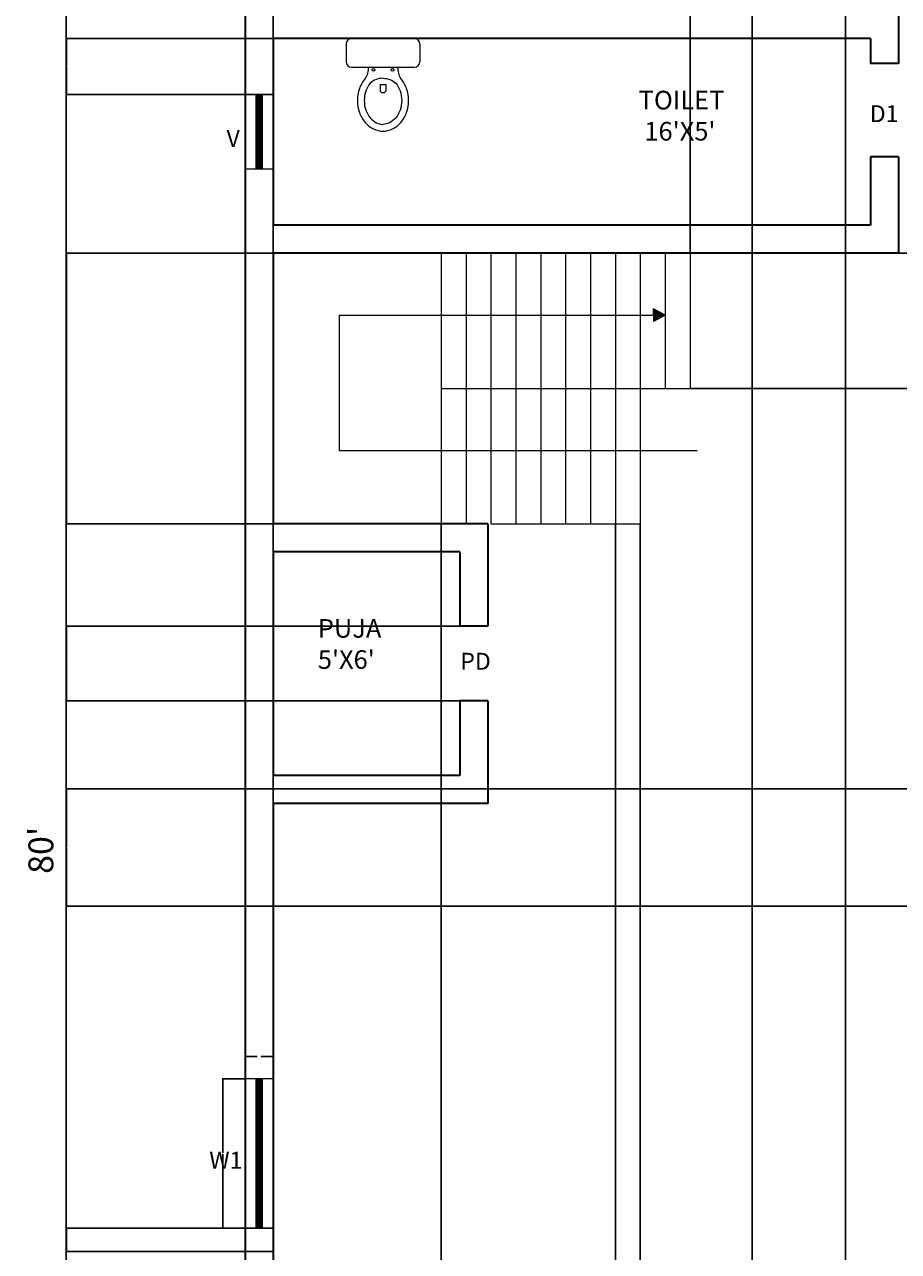
# Model space of a CAD drawing. Units: inches. Extents: x 318 to 927, y -1130 to 13.
# Tile 8 of 17: x 318 to 599, y -692 to -297. Entities that reach past the tile are written whole.
import ezdxf

# ---------------------------------------------------------------- set-up
doc = ezdxf.new("R2010")
doc.units = ezdxf.units.IN
doc.header["$MEASUREMENT"] = 0
for name, color, linetype, lineweight in [('A-ANNO-DIMS', 1, 'Continuous', 18), ('A-ANNO-IDEN', 1, 'Continuous', 13), ('A-ANNO-SYMB', 1, 'Continuous', 13), ('A-AREA-IDEN', 8, 'Continuous', 18), ('A-FLOR-FIXT', 7, 'Continuous', 18), ('A-FLOR-STRS', 1, 'Continuous', 18), ('A-GLAZ-PATT', 5, 'Continuous', 9), ('wall', 1, 'Continuous', 35), ('win', 5, 'Continuous', 18)]:
    doc.layers.add(name, color=color, linetype=linetype, lineweight=lineweight)
doc.styles.get("Standard").update_dxf_attribs({"font": 'arial.ttf'})
doc.dimstyles.get("Standard").update_dxf_attribs({"dimtxt": 0.18, "dimasz": 0.18, "dimexe": 0.18, "dimexo": 0.0625, "dimgap": 0.09, "dimtad": 0, "dimtih": 1, "dimtoh": 1, "dimdec": 1, "dimzin": 0, "dimdsep": 46, "dimlunit": 4, "dimtxsty": 'Standard', "dimcen": 0.09, "dimadec": 0, "dimazin": 0, "dimtfac": 1, "dimtdec": 1, "dimtofl": 0, "dimtmove": 0, "dimatfit": 3, "dimfxl": 1, "dimtolj": 1, "dimtzin": 0, "dimarcsym": 0})

# ---------------------------------------------------------------- blocks, each defined once
blk = doc.blocks.new('WC-P01')
for p, q in [((-230, 0), (230, 0)), ((-270, -40), (-270, -170)), ((270, -40), (270, -170)), ((-230, -210), (230, -210)), ((-111.4, -210), (-111.4, -210)), ((-20, -337.8), (20, -337.8)), ((-20, -337.8), (-20, -385.7)), ((20, -337.8), (20, -385.7)), ((-18.5, -389.3), (-10.5, -397.3)), ((-10.5, -397.3), (10.5, -397.3)), ((10.5, -397.3), (18.5, -389.3))]:
    blk.add_line(p, q)
for points in [[(-111.4, -210, -0.215497), (-132.6, -295.9, 0.09084), (-172.8, -367.1, 0.083285), (-187.5, -455, 0.083285), (-172.8, -542.9, 0.09084), (-132.6, -614.1, 0.104065), (-70, -663.6, 0.115836), (0, -680, 0.115836), (70, -663.6, 0.104065), (132.6, -614.1, 0.09084), (172.8, -542.9, 0.083285), (187.5, -455, 0.083285)], [(-70, -246.4), (-70, -246.4, 0.104065)], [(70, -246.4), (70, -246.4, 0.115836)], [(187.5, -455, 0.083285), (172.8, -367.1, 0.09084), (132.6, -295.9, -0.156524), (111.4, -210)], [(-1.8, -291.3, 0.171753), (-94.2, -327.9, 0.09084), (-125.5, -383.5, 0.083285), (-137.5, -455, 0.083285), (-125.5, -526.5, 0.09084), (-94.2, -582.1, 0.104065), (-47.7, -618.8, 0.115836), (0, -630, 0.115836)], [(1.8, -291.3, -0.171753), (94.2, -327.9, -0.09084), (125.5, -383.5, -0.083285), (137.5, -455, -0.083285), (125.5, -526.5, -0.09084), (94.2, -582.1, -0.104065), (47.7, -618.8, -0.115836), (0, -630, -0.115836)]]:
    blk.add_lwpolyline(points, format="xyb")
for centre in [(-70, -230), (70, -230)]:
    blk.add_circle(centre, 10)
for centre, radius, start, end in [((-230, -40), 40, 90, 180), ((230, -40), 40, 0, 90), ((-230, -170), 40, 180, 270), ((230, -170), 40, 270, 0), ((-15, -385.7), 5, 180, 225), ((15, -385.7), 5, 315, 0)]:
    blk.add_arc(centre, radius, start, end)
blk = doc.blocks.new('_ArchTick')
at = {"color": 0, "linetype": 'ByBlock', "const_width": 0.15}
blk.add_lwpolyline([(-0.5, -0.5), (0.5, 0.5)], dxfattribs=at)
blk = doc.blocks.new('*D4')
at = {"layer": 'A-ANNO-DIMS', "color": 0, "lineweight": -2, "transparency": 16777216}
blk.add_line((331.26, -82.91), (331.26, -1042.91), dxfattribs=at)
at = {"layer": 'Defpoints', "color": 0, "transparency": 16777216}
for p in [(388.89, -82.91), (331.26, -1042.91), (388.89, -1042.91)]:
    blk.add_point(p, dxfattribs=at)
at = {"layer": 'A-ANNO-DIMS', "color": 0, "lineweight": -2, "transparency": 16777216, "xscale": 6, "yscale": 6, "zscale": 6}
for p, rotation in [((331.26, -82.91), 90), ((331.26, -1042.91), 270)]:
    blk.add_blockref('_ArchTick', p, dxfattribs=dict(at, rotation=rotation))
at = {"layer": 'A-ANNO-DIMS', "color": 0, "transparency": 16777216, "insert": (323.18, -562.91), "char_height": 8, "attachment_point": 5, "rotation": 90}
blk.add_mtext("\\A1;80'", dxfattribs=at)
blk = doc.blocks.new('WIN-48IN')
for p, q in [((0, 48), (9, 48)), ((3.5, 48), (3.5, 0)), ((5.5, 48), (5.5, 0)), ((0, 0), (9, 0))]:
    blk.add_line(p, q)
blk = doc.blocks.new('VENT-24IN')
for p, q in [((9, 24), (0, 24)), ((3.5, 0), (3.5, 24)), ((5.5, 0), (5.5, 24)), ((9, 0), (0, 0))]:
    blk.add_line(p, q)
blk = doc.blocks.new('*D19')
at = {"layer": 'A-ANNO-DIMS', "color": 0, "lineweight": -2, "transparency": 16777216}
for p, q in [((388.83, -636.41), (381.51, -636.41)), ((381.69, -636.59), (381.69, -660.23)), ((381.69, -684.23), (381.69, -660.6)), ((388.83, -684.41), (381.51, -684.41))]:
    blk.add_line(p, q, dxfattribs=at)
at = {"layer": 'A-ANNO-DIMS', "color": 0, "transparency": 16777216}
for points in [[(381.66, -636.59), (381.72, -636.59), (381.69, -636.41)], [(381.66, -684.23), (381.72, -684.23), (381.69, -684.41)]]:
    blk.add_solid(points, dxfattribs=at)
at = {"layer": 'Defpoints', "color": 0, "transparency": 16777216}
for p in [(388.89, -636.41), (381.69, -684.41), (388.89, -684.41)]:
    blk.add_point(p, dxfattribs=at)
at = {"layer": 'A-ANNO-DIMS', "color": 0, "transparency": 16777216, "insert": (381.69, -660.41), "char_height": 0.18, "attachment_point": 5}
blk.add_mtext('\\A1;WINDOW W1 4\'-0" TYP.', dxfattribs=at)
blk = doc.blocks.new('*D20')
at = {"layer": 'A-ANNO-DIMS', "color": 0, "lineweight": -2, "transparency": 16777216}
for p, q in [((388.89, -636.35), (388.89, -629.03)), ((389.07, -629.21), (392.76, -629.21)), ((397.71, -629.21), (394.03, -629.21)), ((397.89, -636.35), (397.89, -629.03))]:
    blk.add_line(p, q, dxfattribs=at)
at = {"layer": 'A-ANNO-DIMS', "color": 0, "transparency": 16777216}
for points in [[(389.07, -629.18), (389.07, -629.24), (388.89, -629.21)], [(397.71, -629.18), (397.71, -629.24), (397.89, -629.21)]]:
    blk.add_solid(points, dxfattribs=at)
at = {"layer": 'Defpoints', "color": 0, "transparency": 16777216}
for p in [(388.89, -629.21), (388.89, -636.41), (397.89, -636.41)]:
    blk.add_point(p, dxfattribs=at)
at = {"layer": 'A-ANNO-DIMS', "color": 0, "transparency": 16777216, "insert": (393.39, -629.21), "char_height": 0.18, "attachment_point": 5}
blk.add_mtext('\\A1;0\'-9" TYP.', dxfattribs=at)
blk = doc.blocks.new('*D30')
at = {"layer": 'A-ANNO-DIMS', "color": 0, "lineweight": -2, "transparency": 16777216}
for p, q in [((551.89, -820.85), (551.89, -25.23)), ((552.07, -25.41), (566.56, -25.41)), ((581.71, -25.41), (567.23, -25.41)), ((581.89, -820.85), (581.89, -25.23))]:
    blk.add_line(p, q, dxfattribs=at)
at = {"layer": 'A-ANNO-DIMS', "color": 0, "transparency": 16777216}
for points in [[(552.07, -25.38), (552.07, -25.44), (551.89, -25.41)], [(581.71, -25.38), (581.71, -25.44), (581.89, -25.41)]]:
    blk.add_solid(points, dxfattribs=at)
at = {"layer": 'Defpoints', "color": 0, "transparency": 16777216}
for p in [(581.89, -25.41), (551.89, -820.91), (581.89, -820.91)]:
    blk.add_point(p, dxfattribs=at)
at = {"layer": 'A-ANNO-DIMS', "color": 0, "transparency": 16777216, "insert": (566.89, -25.41), "char_height": 0.18, "attachment_point": 5}
blk.add_mtext('\\A1;2\'-6"', dxfattribs=at)
blk = doc.blocks.new('*D32')
at = {"layer": 'A-ANNO-DIMS', "color": 0, "lineweight": -2, "transparency": 16777216}
for p, q in [((457.83, -490.91), (331.21, -490.91)), ((331.39, -491.09), (331.39, -502.73)), ((331.39, -514.73), (331.39, -503.09)), ((457.83, -514.91), (331.21, -514.91))]:
    blk.add_line(p, q, dxfattribs=at)
at = {"layer": 'A-ANNO-DIMS', "color": 0, "transparency": 16777216}
for points in [[(331.36, -491.09), (331.42, -491.09), (331.39, -490.91)], [(331.36, -514.73), (331.42, -514.73), (331.39, -514.91)]]:
    blk.add_solid(points, dxfattribs=at)
at = {"layer": 'Defpoints', "color": 0, "transparency": 16777216}
for p in [(457.89, -490.91), (331.39, -514.91), (457.89, -514.91)]:
    blk.add_point(p, dxfattribs=at)
at = {"layer": 'A-ANNO-DIMS', "color": 0, "transparency": 16777216, "insert": (331.39, -502.91), "char_height": 0.18, "attachment_point": 5}
blk.add_mtext('\\A1;2\'-0"', dxfattribs=at)
blk = doc.blocks.new('*D33')
at = {"layer": 'A-ANNO-DIMS', "color": 0, "lineweight": -2, "transparency": 16777216}
for p, q in [((397.89, -370.85), (397.89, -25.23)), ((398.07, -25.41), (464.5, -25.41)), ((531.71, -25.41), (465.28, -25.41)), ((531.89, -370.85), (531.89, -25.23))]:
    blk.add_line(p, q, dxfattribs=at)
at = {"layer": 'A-ANNO-DIMS', "color": 0, "transparency": 16777216}
for points in [[(398.07, -25.38), (398.07, -25.44), (397.89, -25.41)], [(531.71, -25.38), (531.71, -25.44), (531.89, -25.41)]]:
    blk.add_solid(points, dxfattribs=at)
at = {"layer": 'Defpoints', "color": 0, "transparency": 16777216}
for p in [(531.89, -25.41), (397.89, -370.91), (531.89, -370.91)]:
    blk.add_point(p, dxfattribs=at)
at = {"layer": 'A-ANNO-DIMS', "color": 0, "transparency": 16777216, "insert": (464.89, -25.41), "char_height": 0.18, "attachment_point": 5}
blk.add_mtext('\\A1;11\'-2"', dxfattribs=at)
blk = doc.blocks.new('*D34')
at = {"layer": 'A-ANNO-DIMS', "color": 0, "lineweight": -2, "transparency": 16777216}
for p, q in [((397.83, -370.91), (331.21, -370.91)), ((331.39, -371.09), (331.39, -414.23)), ((331.39, -457.73), (331.39, -414.59)), ((397.83, -457.91), (331.21, -457.91))]:
    blk.add_line(p, q, dxfattribs=at)
at = {"layer": 'A-ANNO-DIMS', "color": 0, "transparency": 16777216}
for points in [[(331.36, -371.09), (331.42, -371.09), (331.39, -370.91)], [(331.36, -457.73), (331.42, -457.73), (331.39, -457.91)]]:
    blk.add_solid(points, dxfattribs=at)
at = {"layer": 'Defpoints', "color": 0, "transparency": 16777216}
for p in [(397.89, -370.91), (331.39, -457.91), (397.89, -457.91)]:
    blk.add_point(p, dxfattribs=at)
at = {"layer": 'A-ANNO-DIMS', "color": 0, "transparency": 16777216, "insert": (331.39, -414.41), "char_height": 0.18, "attachment_point": 5}
blk.add_mtext('\\A1;7\'-3"', dxfattribs=at)
blk = doc.blocks.new('*D35')
at = {"layer": 'A-ANNO-DIMS', "color": 0, "lineweight": -2, "transparency": 16777216}
for p, q in [((397.89, -457.98), (397.89, -1124.59)), ((451.89, -457.98), (451.89, -1124.59)), ((398.07, -1124.41), (424.56, -1124.41)), ((451.71, -1124.41), (425.23, -1124.41))]:
    blk.add_line(p, q, dxfattribs=at)
at = {"layer": 'A-ANNO-DIMS', "color": 0, "transparency": 16777216}
for points in [[(398.07, -1124.38), (398.07, -1124.44), (397.89, -1124.41)], [(451.71, -1124.38), (451.71, -1124.44), (451.89, -1124.41)]]:
    blk.add_solid(points, dxfattribs=at)
at = {"layer": 'Defpoints', "color": 0, "transparency": 16777216}
for p in [(397.89, -457.91), (451.89, -457.91), (451.89, -1124.41)]:
    blk.add_point(p, dxfattribs=at)
at = {"layer": 'A-ANNO-DIMS', "color": 0, "transparency": 16777216, "insert": (424.89, -1124.41), "char_height": 0.18, "attachment_point": 5}
blk.add_mtext('\\A1;4\'-6"', dxfattribs=at)
blk = doc.blocks.new('*D36')
at = {"layer": 'A-ANNO-DIMS', "color": 0, "lineweight": -2, "transparency": 16777216}
for p, q in [((507.89, -457.98), (507.89, -1124.59)), ((515.89, -457.98), (515.89, -1124.59)), ((508.07, -1124.41), (511.57, -1124.41)), ((515.71, -1124.41), (512.22, -1124.41))]:
    blk.add_line(p, q, dxfattribs=at)
at = {"layer": 'A-ANNO-DIMS', "color": 0, "transparency": 16777216}
for points in [[(508.07, -1124.38), (508.07, -1124.44), (507.89, -1124.41)], [(515.71, -1124.38), (515.71, -1124.44), (515.89, -1124.41)]]:
    blk.add_solid(points, dxfattribs=at)
at = {"layer": 'Defpoints', "color": 0, "transparency": 16777216}
for p in [(507.89, -457.91), (515.89, -457.91), (515.89, -1124.41)]:
    blk.add_point(p, dxfattribs=at)
at = {"layer": 'A-ANNO-DIMS', "color": 0, "transparency": 16777216, "insert": (511.89, -1124.41), "char_height": 0.18, "attachment_point": 5}
blk.add_mtext('\\A1;0\'-8"', dxfattribs=at)
blk = doc.blocks.new('*D37')
at = {"layer": 'A-ANNO-DIMS', "color": 0, "lineweight": -2, "transparency": 16777216}
for p, q in [((531.96, -370.91), (926.57, -370.91)), ((926.39, -371.09), (926.39, -392.48)), ((926.39, -414.23), (926.39, -392.85)), ((531.96, -414.41), (926.57, -414.41))]:
    blk.add_line(p, q, dxfattribs=at)
at = {"layer": 'A-ANNO-DIMS', "color": 0, "transparency": 16777216}
for points in [[(926.36, -371.09), (926.42, -371.09), (926.39, -370.91)], [(926.36, -414.23), (926.42, -414.23), (926.39, -414.41)]]:
    blk.add_solid(points, dxfattribs=at)
at = {"layer": 'Defpoints', "color": 0, "transparency": 16777216}
for p in [(531.89, -370.91), (531.89, -414.41), (926.39, -414.41)]:
    blk.add_point(p, dxfattribs=at)
at = {"layer": 'A-ANNO-DIMS', "color": 0, "transparency": 16777216, "insert": (926.39, -392.66), "char_height": 0.18, "attachment_point": 5}
blk.add_mtext('\\A1;3\'-7 1/2"', dxfattribs=at)
blk = doc.blocks.new('*D41')
at = {"layer": 'A-ANNO-DIMS', "color": 0, "lineweight": -2, "transparency": 16777216}
for p, q in [((790.59, -543.15), (331.21, -543.15)), ((331.39, -543.33), (331.39, -561.86)), ((331.39, -580.75), (331.39, -562.22)), ((790.59, -580.93), (331.21, -580.93))]:
    blk.add_line(p, q, dxfattribs=at)
at = {"layer": 'A-ANNO-DIMS', "color": 0, "transparency": 16777216}
for points in [[(331.36, -543.33), (331.42, -543.33), (331.39, -543.15)], [(331.36, -580.75), (331.42, -580.75), (331.39, -580.93)]]:
    blk.add_solid(points, dxfattribs=at)
at = {"layer": 'Defpoints', "color": 0, "transparency": 16777216}
for p in [(790.65, -543.15), (331.39, -580.93), (790.65, -580.93)]:
    blk.add_point(p, dxfattribs=at)
at = {"layer": 'A-ANNO-DIMS', "color": 0, "transparency": 16777216, "insert": (331.39, -562.04), "char_height": 0.18, "attachment_point": 5}
blk.add_mtext('\\A1;3\'-2"', dxfattribs=at)
blk = doc.blocks.new('*D67')
at = {"layer": 'A-ANNO-DIMS', "color": 0, "lineweight": -2, "transparency": 16777216}
for p, q in [((397.83, -301.91), (331.21, -301.91)), ((331.39, -302.09), (331.39, -310.73)), ((331.39, -319.73), (331.39, -311.09)), ((397.83, -319.91), (331.21, -319.91))]:
    blk.add_line(p, q, dxfattribs=at)
at = {"layer": 'A-ANNO-DIMS', "color": 0, "transparency": 16777216}
for points in [[(331.36, -302.09), (331.42, -302.09), (331.39, -301.91)], [(331.36, -319.73), (331.42, -319.73), (331.39, -319.91)]]:
    blk.add_solid(points, dxfattribs=at)
at = {"layer": 'Defpoints', "color": 0, "transparency": 16777216}
for p in [(397.89, -301.91), (331.39, -319.91), (397.89, -319.91)]:
    blk.add_point(p, dxfattribs=at)
at = {"layer": 'A-ANNO-DIMS', "color": 0, "transparency": 16777216, "insert": (331.39, -310.91), "char_height": 0.18, "attachment_point": 5}
blk.add_mtext('\\A1;1\'-6"', dxfattribs=at)
blk = doc.blocks.new('*D68')
at = {"layer": 'A-ANNO-DIMS', "color": 0, "lineweight": -2, "transparency": 16777216}
for p, q in [((397.83, -684.41), (331.21, -684.41)), ((331.39, -684.59), (331.39, -687.98)), ((331.39, -691.73), (331.39, -688.35)), ((397.83, -691.91), (331.21, -691.91))]:
    blk.add_line(p, q, dxfattribs=at)
at = {"layer": 'A-ANNO-DIMS', "color": 0, "transparency": 16777216}
for points in [[(331.36, -684.59), (331.42, -684.59), (331.39, -684.41)], [(331.36, -691.73), (331.42, -691.73), (331.39, -691.91)]]:
    blk.add_solid(points, dxfattribs=at)
at = {"layer": 'Defpoints', "color": 0, "transparency": 16777216}
for p in [(331.39, -684.41), (397.89, -684.41), (397.89, -691.91)]:
    blk.add_point(p, dxfattribs=at)
at = {"layer": 'A-ANNO-DIMS', "color": 0, "transparency": 16777216, "insert": (331.39, -688.16), "char_height": 0.18, "attachment_point": 5}
blk.add_mtext('\\A1;0\'-7 1/2"', dxfattribs=at)

msp = doc.modelspace()

# ---------------------------------------------------------------- hatches: boundary and pattern name
at = {"layer": 'A-ANNO-SYMB'}
h = msp.add_hatch(dxfattribs=at)
h.set_pattern_fill('ANSI31', color=256)
h.paths.add_polyline_path([(520.1, -388.85), (520.1, -390.85), (520.1, -392.85), (523.89, -390.85)])
at = {"layer": 'A-GLAZ-PATT'}
h = msp.add_hatch(dxfattribs=at)
h.set_pattern_fill('ANSI31', color=256)
h.paths.add_polyline_path([(394.39, -636.41), (392.39, -636.41), (392.39, -684.41), (394.39, -684.41)])
h.paths.add_polyline_path([(394.39, -319.91), (392.39, -319.91), (392.39, -343.91), (394.39, -343.91)])
h.paths.add_polyline_path([(394.39, -172.63), (392.39, -172.63), (392.39, -208.63), (394.39, -208.63)])
h.paths.add_polyline_path([(394.39, -109.91), (392.39, -109.91), (392.39, -133.91), (394.39, -133.91)])
h.paths.add_polyline_path([(865.39, -102.49), (863.39, -102.49), (863.39, -138.49), (865.39, -138.49)])

# ---------------------------------------------------------------- linework, layer by layer
at = {"layer": 'A-ANNO-SYMB'}
for p, q in [((520.1, -390.85), (520.1, -388.85)), ((523.89, -390.85), (520.1, -388.85)), ((419.22, -434.49), (419.22, -390.85)), ((419.22, -390.85), (520.1, -390.85)), ((520.1, -390.85), (520.1, -392.85)), ((523.89, -390.85), (520.1, -392.85)), ((534.23, -434.49), (419.22, -434.49))]:
    msp.add_line(p, q, dxfattribs=at)
at = {"layer": 'A-FLOR-STRS'}
for p, q in [((451.89, -370.91), (451.89, -457.91)), ((459.89, -370.91), (459.89, -457.91)), ((467.89, -370.91), (467.89, -457.91)), ((475.89, -370.91), (475.89, -457.91)), ((483.89, -370.91), (483.89, -457.91)), ((491.89, -370.91), (491.89, -457.91)), ((499.89, -370.91), (499.89, -457.91)), ((507.89, -370.91), (507.89, -457.91)), ((515.89, -370.91), (515.89, -457.91)), ((523.89, -370.91), (523.89, -414.41)), ((531.89, -370.91), (531.89, -414.41)), ((451.89, -414.41), (531.89, -414.41)), ((467.89, -457.91), (515.89, -457.91))]:
    msp.add_line(p, q, dxfattribs=at)
at = {"layer": 'wall'}
for p, q in [((388.89, -82.91), (388.89, -1042.91)), ((598.89, -204.91), (598.89, -309.91)), ((589.89, -301.91), (397.89, -301.91)), ((589.89, -301.91), (397.89, -301.91)), ((397.89, -301.91), (397.89, -361.91)), ((589.89, -301.91), (589.89, -309.91)), ((598.89, -309.91), (589.89, -309.91)), ((598.89, -339.91), (589.89, -339.91)), ((589.89, -339.91), (589.89, -361.91)), ((598.89, -339.91), (598.89, -370.91)), ((589.89, -361.91), (397.89, -361.91)), ((598.89, -370.91), (397.89, -370.91)), ((397.89, -370.91), (397.89, -457.91)), ((466.89, -457.91), (397.89, -457.91)), ((466.89, -457.91), (466.89, -490.91)), ((457.89, -466.91), (397.89, -466.91)), ((397.89, -466.91), (397.89, -538.91)), ((457.89, -466.91), (457.89, -490.91)), ((466.89, -490.91), (457.89, -490.91)), ((466.89, -514.91), (457.89, -514.91)), ((457.89, -514.91), (457.89, -538.91)), ((466.89, -514.91), (466.89, -547.91)), ((457.89, -538.91), (397.89, -538.91)), ((466.89, -547.91), (397.89, -547.91)), ((397.89, -547.91), (397.89, -820.91))]:
    msp.add_line(p, q, dxfattribs=at)

# ---------------------------------------------------------------- block references
at = {"layer": 'A-FLOR-FIXT', "xscale": 0.0438047028060103, "yscale": 0.0438047028060103, "zscale": 0.0438047028060103}
msp.add_blockref('WC-P01', (433.17, -301.91), dxfattribs=at)
at = {"layer": 'win'}
msp.add_blockref('VENT-24IN', (388.89, -343.91), dxfattribs=at)
at = {"layer": 'win', "rotation": 180}
msp.add_blockref('WIN-48IN', (397.89, -636.41), dxfattribs=at)

# ---------------------------------------------------------------- texts
at = {"layer": 'A-ANNO-IDEN'}
for s, height, p in [('D1', 5.444, (589.67, -328.79)), ('V', 5.44, (382.87, -336.76)), ('PD', 5.444, (458.02, -504.87)), ('W1', 5.444, (377.33, -665.31))]:
    msp.add_text(s, height=height, dxfattribs=at).set_placement(p)
at = {"layer": 'A-AREA-IDEN', "char_height": 6, "attachment_point": 1}
for s, width, insert in [(" TOILET\\P  16'X5'", 32.6904, (513.54, -318.71)), ("PUJA\\P5'X6'", 24.4662, (412.22, -488.58))]:
    msp.add_mtext_dynamic_manual_height_columns(s, width=width, gutter_width=1, heights=[0], dxfattribs=dict(at, insert=insert))

# ---------------------------------------------------------------- dimensions: what is measured, and where the dimension line sits
at = {"layer": 'A-ANNO-DIMS'}
for base, p1, p2, picture, middle in [((531.89, -25.41), (397.89, -370.91), (531.89, -370.91), '*D33', (464.89, -25.41)), ((581.89, -25.41), (551.89, -820.91), (581.89, -820.91), '*D30', (566.89, -25.41)), ((451.89, -1124.41), (397.89, -457.91), (451.89, -457.91), '*D35', (424.89, -1124.41)), ((515.89, -1124.41), (507.89, -457.91), (515.89, -457.91), '*D36', (511.89, -1124.41))]:
    dim = msp.add_linear_dim(base=base, p1=p1, p2=p2, dimstyle='Standard', override={"dimdec": 1, "dimlfac": 1, "dimrnd": 0, "dimzin": 1, "dimdsep": 46, "dimlunit": 4, "dimfrac": 2}, dxfattribs=at)
    dim.commit()
    dim.dimension.update_dxf_attribs({"geometry": picture, "text_midpoint": middle})
for base, p1, p2, override, picture, middle in [((331.26, -1042.91), (388.89, -82.91), (388.89, -1042.91), {"dimtxt": 8, "dimasz": 6, "dimgap": 4, "dimtad": 1, "dimtih": 0, "dimblk1": 'ArchTick', "dimblk2": 'ArchTick', "dimsah": 1, "dimse1": 1, "dimse2": 1, "dimclrd": 0, "dimclre": 0, "dimclrt": 0}, '*D4', (323.18, -562.91)), ((331.39, -319.91), (397.89, -301.91), (397.89, -319.91), {"dimdec": 1, "dimlfac": 1, "dimrnd": 0, "dimzin": 1, "dimdsep": 46, "dimlunit": 4, "dimfrac": 2}, '*D67', (331.39, -310.91)), ((331.39, -457.91), (397.89, -370.91), (397.89, -457.91), {"dimdec": 1, "dimlfac": 1, "dimrnd": 0, "dimzin": 1, "dimdsep": 46, "dimlunit": 4, "dimfrac": 2}, '*D34', (331.39, -414.41)), ((926.39, -414.41), (531.89, -370.91), (531.89, -414.41), {"dimdec": 1, "dimlfac": 1, "dimrnd": 0, "dimzin": 1, "dimdsep": 46, "dimlunit": 4, "dimfrac": 2}, '*D37', (926.39, -392.66)), ((331.39, -514.91), (457.89, -490.91), (457.89, -514.91), {"dimdec": 1, "dimlfac": 1, "dimrnd": 0, "dimzin": 1, "dimdsep": 46, "dimlunit": 4, "dimfrac": 2}, '*D32', (331.39, -502.91)), ((331.39, -580.93), (790.65, -543.15), (790.65, -580.93), {"dimdec": 1, "dimlfac": 1, "dimrnd": 0, "dimzin": 1, "dimdsep": 46, "dimlunit": 4, "dimfrac": 2}, '*D41', (331.39, -562.04)), ((331.39, -684.41), (397.89, -691.91), (397.89, -684.41), {"dimdec": 1, "dimlfac": 1, "dimrnd": 0, "dimzin": 1, "dimdsep": 46, "dimlunit": 4, "dimfrac": 2}, '*D68', (331.39, -688.16))]:
    dim = msp.add_linear_dim(base=base, p1=p1, p2=p2, angle=90, dimstyle='Standard', override=override, dxfattribs=at)
    dim.commit()
    dim.dimension.update_dxf_attribs({"geometry": picture, "text_midpoint": middle})
for base, p1, p2, angle, text, picture, middle in [((388.89, -629.21), (397.89, -636.41), (388.89, -636.41), 180, '<> TYP.', '*D20', (393.39, -629.21)), ((381.69, -684.41), (388.89, -636.41), (388.89, -684.41), 270, 'WINDOW W1 <> TYP.', '*D19', (381.69, -660.41))]:
    dim = msp.add_linear_dim(base=base, p1=p1, p2=p2, angle=angle, text=text, dimstyle='Standard', override={"dimdec": 1, "dimlfac": 1, "dimrnd": 0, "dimzin": 1, "dimdsep": 46, "dimlunit": 4, "dimfrac": 2}, dxfattribs=at)
    dim.commit()
    dim.dimension.update_dxf_attribs({"geometry": picture, "text_midpoint": middle})

doc.saveas('drawing.dxf')
